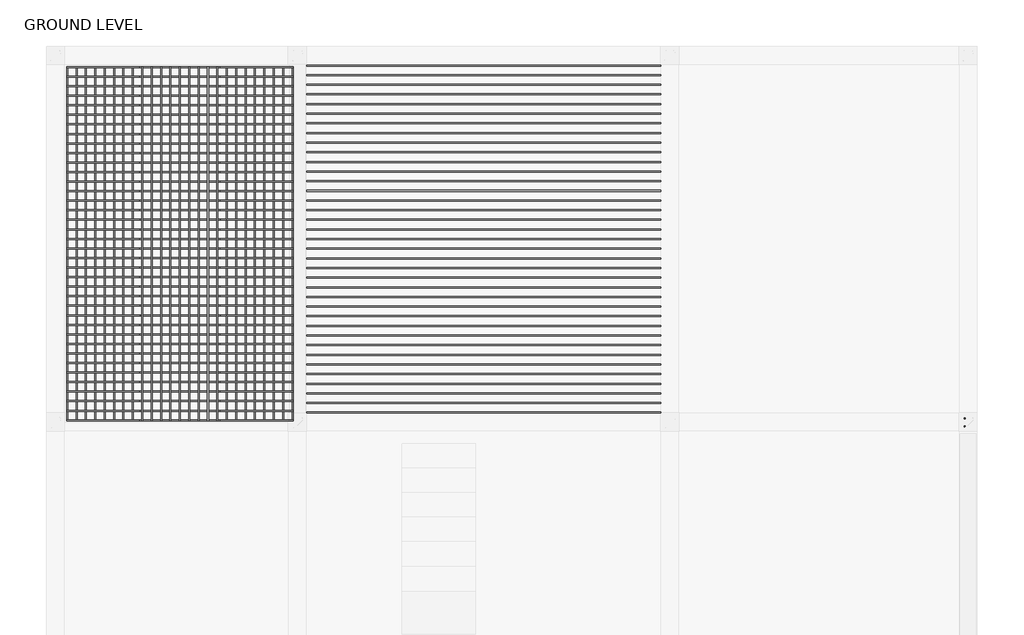
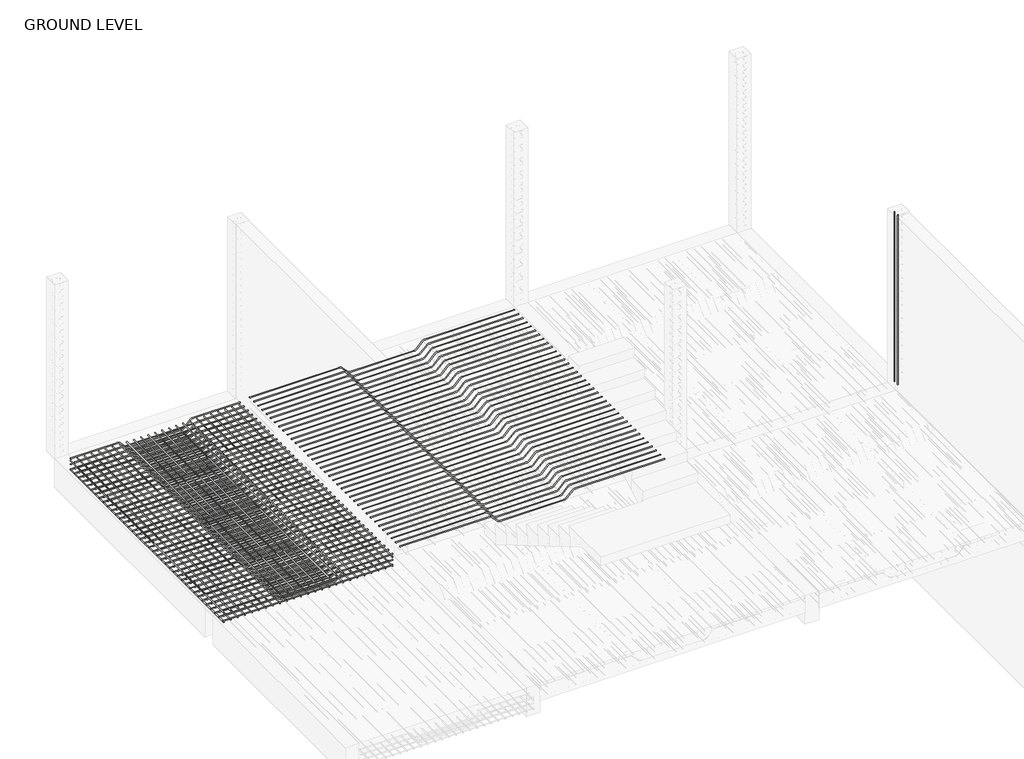
# One storey, part 6 of 8: 7 reinforcing bars.
"""IFC4 building model written with IfcOpenShell, lengths in millimetres."""

from ifc_helpers import new_model, si_unit, point, frame, origin, place, context, project, spatial, polyline, circle_curve, trimmed, segment, composite_curve, source, transform, mapped, element, save
from ifc_brep_helpers import swept_disk

model = new_model("IFC4")

# Units and contexts
model_context = context("Model", 3, world=origin())
ifc_project = project(units=[si_unit("LENGTHUNIT", "METRE", prefix="MILLI")], contexts=[model_context])

# Site, building, storey
site = spatial("IfcSite", under=ifc_project)
building = spatial("IfcBuilding", under=site)
storey = spatial("IfcBuildingStorey", under=building, Name="GROUND LEVEL", Elevation=0.0)

# Reinforcing bars
placement = place(None, origin())
reinforcing_bar_shape = source(origin(), model_context, "Body", "SolidModel", [
    swept_disk(composite_curve([segment(polyline([(-14789.4556799, 4171.9516651, -60.0), (-14008.6544785, 4171.9516651, -60.0)]), True, "CONTINUOUS"), segment(trimmed(circle_curve(frame((-14008.6544785, 4171.9516651, -106.35), z_axis=(0.0, 1.0, 0.0), x_axis=(0.0, 0.0, 46.349999999999994)), 46.35), [point((-14008.6544785, 4171.9516651, -60.0))], [point((-13975.8800792, 4171.9516651, -73.5756007))], True, "CARTESIAN"), True, "CONTINUOUS"), segment(polyline([(-13975.8800792, 4171.9516651, -73.5756007), (-13861.6099243, 4171.9516651, -187.8457555)]), True, "CONTINUOUS"), segment(trimmed(circle_curve(frame((-13828.835525, 4171.9516651, -155.0713562), z_axis=(0.0, -1.0, 0.0), x_axis=(-32.77439930000037, 0.0, -32.7743993)), 46.35), [point((-13861.6099243, 4171.9516651, -187.8457555))], [point((-13828.835525, 4171.9516651, -201.4213562))], True, "CARTESIAN"), True, "CONTINUOUS"), segment(polyline([(-13828.835525, 4171.9516651, -201.4213562), (-12945.2758347, 4171.9516651, -201.4213562)]), True, "CONTINUOUS"), segment(trimmed(circle_curve(frame((-12945.2758347, 4171.9516651, -155.0713562), z_axis=(0.0, -1.0, 0.0), x_axis=(0.0, 0.0, -46.349999999999994)), 46.35), [point((-12945.2758347, 4171.9516651, -201.4213562))], [point((-12912.5014354, 4171.9516651, -187.8457555))], True, "CARTESIAN"), True, "CONTINUOUS"), segment(polyline([(-12912.5014354, 4171.9516651, -187.8457555), (-12798.2312806, 4171.9516651, -73.5756007)]), True, "CONTINUOUS"), segment(trimmed(circle_curve(frame((-12765.4568813, 4171.9516651, -106.35), z_axis=(0.0, 1.0000000000000002, 0.0), x_axis=(-32.77439930000037, 0.0, 32.7743993)), 46.35), [point((-12798.2312806, 4171.9516651, -73.5756007))], [point((-12765.4568813, 4171.9516651, -60.0))], True, "CARTESIAN"), True, "CONTINUOUS"), segment(polyline([(-12765.4568813, 4171.9516651, -60.0), (-11984.6556799, 4171.9516651, -60.0)]), True, "CONTINUOUS")], self_intersect=False), 6.35),
])
element("IfcReinforcingBar", 1, at=placement, inside=storey, context=model_context, shape_type="MappedRepresentation", body=[
    mapped(reinforcing_bar_shape, transform((0.0, 0.0, 0.0), x_axis=(1.0, 0.0, 0.0), y_axis=(0.0, 1.0, 0.0), z_axis=(0.0, 0.0, 1.0))),
    mapped(reinforcing_bar_shape, transform((0.0, -118.3325458, 0.0), x_axis=(1.0, 0.0, 0.0), y_axis=(0.0, 1.0, 0.0), z_axis=(0.0, 0.0, 1.0))),
    mapped(reinforcing_bar_shape, transform((0.0, -236.6650915, 0.0), x_axis=(1.0, 0.0, 0.0), y_axis=(0.0, 1.0, 0.0), z_axis=(0.0, 0.0, 1.0))),
    mapped(reinforcing_bar_shape, transform((0.0, -354.9976373, 0.0), x_axis=(1.0, 0.0, 0.0), y_axis=(0.0, 1.0, 0.0), z_axis=(0.0, 0.0, 1.0))),
    mapped(reinforcing_bar_shape, transform((0.0, -473.330183, 0.0), x_axis=(1.0, 0.0, 0.0), y_axis=(0.0, 1.0, 0.0), z_axis=(0.0, 0.0, 1.0))),
    mapped(reinforcing_bar_shape, transform((0.0, -591.6627288, 0.0), x_axis=(1.0, 0.0, 0.0), y_axis=(0.0, 1.0, 0.0), z_axis=(0.0, 0.0, 1.0))),
    mapped(reinforcing_bar_shape, transform((0.0, -709.9952745, 0.0), x_axis=(1.0, 0.0, 0.0), y_axis=(0.0, 1.0, 0.0), z_axis=(0.0, 0.0, 1.0))),
    mapped(reinforcing_bar_shape, transform((0.0, -828.3278203, 0.0), x_axis=(1.0, 0.0, 0.0), y_axis=(0.0, 1.0, 0.0), z_axis=(0.0, 0.0, 1.0))),
    mapped(reinforcing_bar_shape, transform((0.0, -946.660366, 0.0), x_axis=(1.0, 0.0, 0.0), y_axis=(0.0, 1.0, 0.0), z_axis=(0.0, 0.0, 1.0))),
    mapped(reinforcing_bar_shape, transform((0.0, -1064.9929118, 0.0), x_axis=(1.0, 0.0, 0.0), y_axis=(0.0, 1.0, 0.0), z_axis=(0.0, 0.0, 1.0))),
    mapped(reinforcing_bar_shape, transform((0.0, -1183.3254576, 0.0), x_axis=(1.0, 0.0, 0.0), y_axis=(0.0, 1.0, 0.0), z_axis=(0.0, 0.0, 1.0))),
    mapped(reinforcing_bar_shape, transform((0.0, -1301.6580033, 0.0), x_axis=(1.0, 0.0, 0.0), y_axis=(0.0, 1.0, 0.0), z_axis=(0.0, 0.0, 1.0))),
    mapped(reinforcing_bar_shape, transform((0.0, -1419.9905491, 0.0), x_axis=(1.0, 0.0, 0.0), y_axis=(0.0, 1.0, 0.0), z_axis=(0.0, 0.0, 1.0))),
    mapped(reinforcing_bar_shape, transform((0.0, -1538.3230948, 0.0), x_axis=(1.0, 0.0, 0.0), y_axis=(0.0, 1.0, 0.0), z_axis=(0.0, 0.0, 1.0))),
    mapped(reinforcing_bar_shape, transform((0.0, -1656.6556406, 0.0), x_axis=(1.0, 0.0, 0.0), y_axis=(0.0, 1.0, 0.0), z_axis=(0.0, 0.0, 1.0))),
    mapped(reinforcing_bar_shape, transform((0.0, -1774.9881863, 0.0), x_axis=(1.0, 0.0, 0.0), y_axis=(0.0, 1.0, 0.0), z_axis=(0.0, 0.0, 1.0))),
    mapped(reinforcing_bar_shape, transform((0.0, -1893.3207321, 0.0), x_axis=(1.0, 0.0, 0.0), y_axis=(0.0, 1.0, 0.0), z_axis=(0.0, 0.0, 1.0))),
    mapped(reinforcing_bar_shape, transform((0.0, -2011.6532778, 0.0), x_axis=(1.0, 0.0, 0.0), y_axis=(0.0, 1.0, 0.0), z_axis=(0.0, 0.0, 1.0))),
    mapped(reinforcing_bar_shape, transform((0.0, -2129.9858236, 0.0), x_axis=(1.0, 0.0, 0.0), y_axis=(0.0, 1.0, 0.0), z_axis=(0.0, 0.0, 1.0))),
    mapped(reinforcing_bar_shape, transform((0.0, -2248.3183694, 0.0), x_axis=(1.0, 0.0, 0.0), y_axis=(0.0, 1.0, 0.0), z_axis=(0.0, 0.0, 1.0))),
    mapped(reinforcing_bar_shape, transform((0.0, -2366.6509151, 0.0), x_axis=(1.0, 0.0, 0.0), y_axis=(0.0, 1.0, 0.0), z_axis=(0.0, 0.0, 1.0))),
    mapped(reinforcing_bar_shape, transform((0.0, -2484.9834609, 0.0), x_axis=(1.0, 0.0, 0.0), y_axis=(0.0, 1.0, 0.0), z_axis=(0.0, 0.0, 1.0))),
    mapped(reinforcing_bar_shape, transform((0.0, -2603.3160066, 0.0), x_axis=(1.0, 0.0, 0.0), y_axis=(0.0, 1.0, 0.0), z_axis=(0.0, 0.0, 1.0))),
    mapped(reinforcing_bar_shape, transform((0.0, -2721.6485524, 0.0), x_axis=(1.0, 0.0, 0.0), y_axis=(0.0, 1.0, 0.0), z_axis=(0.0, 0.0, 1.0))),
    mapped(reinforcing_bar_shape, transform((0.0, -2839.9810981, 0.0), x_axis=(1.0, 0.0, 0.0), y_axis=(0.0, 1.0, 0.0), z_axis=(0.0, 0.0, 1.0))),
    mapped(reinforcing_bar_shape, transform((0.0, -2958.3136439, 0.0), x_axis=(1.0, 0.0, 0.0), y_axis=(0.0, 1.0, 0.0), z_axis=(0.0, 0.0, 1.0))),
    mapped(reinforcing_bar_shape, transform((0.0, -3076.6461896, 0.0), x_axis=(1.0, 0.0, 0.0), y_axis=(0.0, 1.0, 0.0), z_axis=(0.0, 0.0, 1.0))),
    mapped(reinforcing_bar_shape, transform((0.0, -3194.9787354, 0.0), x_axis=(1.0, 0.0, 0.0), y_axis=(0.0, 1.0, 0.0), z_axis=(0.0, 0.0, 1.0))),
    mapped(reinforcing_bar_shape, transform((0.0, -3313.3112812, 0.0), x_axis=(1.0, 0.0, 0.0), y_axis=(0.0, 1.0, 0.0), z_axis=(0.0, 0.0, 1.0))),
    mapped(reinforcing_bar_shape, transform((0.0, -3431.6438269, 0.0), x_axis=(1.0, 0.0, 0.0), y_axis=(0.0, 1.0, 0.0), z_axis=(0.0, 0.0, 1.0))),
    mapped(reinforcing_bar_shape, transform((0.0, -3549.9763727, 0.0), x_axis=(1.0, 0.0, 0.0), y_axis=(0.0, 1.0, 0.0), z_axis=(0.0, 0.0, 1.0))),
    mapped(reinforcing_bar_shape, transform((0.0, -3668.3089184, 0.0), x_axis=(1.0, 0.0, 0.0), y_axis=(0.0, 1.0, 0.0), z_axis=(0.0, 0.0, 1.0))),
    mapped(reinforcing_bar_shape, transform((0.0, -3786.6414642, 0.0), x_axis=(1.0, 0.0, 0.0), y_axis=(0.0, 1.0, 0.0), z_axis=(0.0, 0.0, 1.0))),
    mapped(reinforcing_bar_shape, transform((0.0, -3904.9740099, 0.0), x_axis=(1.0, 0.0, 0.0), y_axis=(0.0, 1.0, 0.0), z_axis=(0.0, 0.0, 1.0))),
    mapped(reinforcing_bar_shape, transform((0.0, -4023.3065557, 0.0), x_axis=(1.0, 0.0, 0.0), y_axis=(0.0, 1.0, 0.0), z_axis=(0.0, 0.0, 1.0))),
    mapped(reinforcing_bar_shape, transform((0.0, -4141.6391014, 0.0), x_axis=(1.0, 0.0, 0.0), y_axis=(0.0, 1.0, 0.0), z_axis=(0.0, 0.0, 1.0))),
    mapped(reinforcing_bar_shape, transform((0.0, -4259.9716472, 0.0), x_axis=(1.0, 0.0, 0.0), y_axis=(0.0, 1.0, 0.0), z_axis=(0.0, 0.0, 1.0))),
    mapped(reinforcing_bar_shape, transform((0.0, -4378.304193, 0.0), x_axis=(1.0, 0.0, 0.0), y_axis=(0.0, 1.0, 0.0), z_axis=(0.0, 0.0, 1.0))),
])
reinforcing_bar_2_shape = source(origin(), model_context, "Body", "SolidModel", [
    swept_disk(composite_curve([segment(polyline([(-11984.6556799, 4171.9516651, -249.9712592), (-14789.4556799, 4171.9516651, -249.9712592)]), True, "CONTINUOUS")], self_intersect=False), 6.35),
])
element("IfcReinforcingBar", 2, at=placement, inside=storey, context=model_context, shape_type="MappedRepresentation", body=[
    mapped(reinforcing_bar_2_shape, transform((0.0, 0.0, 0.0), x_axis=(1.0, 0.0, 0.0), y_axis=(0.0, 1.0, 0.0), z_axis=(0.0, 0.0, 1.0))),
    mapped(reinforcing_bar_2_shape, transform((0.0, -118.3325458, 0.0), x_axis=(1.0, 0.0, 0.0), y_axis=(0.0, 1.0, 0.0), z_axis=(0.0, 0.0, 1.0))),
    mapped(reinforcing_bar_2_shape, transform((0.0, -236.6650915, 0.0), x_axis=(1.0, 0.0, 0.0), y_axis=(0.0, 1.0, 0.0), z_axis=(0.0, 0.0, 1.0))),
    mapped(reinforcing_bar_2_shape, transform((0.0, -354.9976373, 0.0), x_axis=(1.0, 0.0, 0.0), y_axis=(0.0, 1.0, 0.0), z_axis=(0.0, 0.0, 1.0))),
    mapped(reinforcing_bar_2_shape, transform((0.0, -473.330183, 0.0), x_axis=(1.0, 0.0, 0.0), y_axis=(0.0, 1.0, 0.0), z_axis=(0.0, 0.0, 1.0))),
    mapped(reinforcing_bar_2_shape, transform((0.0, -591.6627288, 0.0), x_axis=(1.0, 0.0, 0.0), y_axis=(0.0, 1.0, 0.0), z_axis=(0.0, 0.0, 1.0))),
    mapped(reinforcing_bar_2_shape, transform((0.0, -709.9952745, 0.0), x_axis=(1.0, 0.0, 0.0), y_axis=(0.0, 1.0, 0.0), z_axis=(0.0, 0.0, 1.0))),
    mapped(reinforcing_bar_2_shape, transform((0.0, -828.3278203, 0.0), x_axis=(1.0, 0.0, 0.0), y_axis=(0.0, 1.0, 0.0), z_axis=(0.0, 0.0, 1.0))),
    mapped(reinforcing_bar_2_shape, transform((0.0, -946.660366, 0.0), x_axis=(1.0, 0.0, 0.0), y_axis=(0.0, 1.0, 0.0), z_axis=(0.0, 0.0, 1.0))),
    mapped(reinforcing_bar_2_shape, transform((0.0, -1064.9929118, 0.0), x_axis=(1.0, 0.0, 0.0), y_axis=(0.0, 1.0, 0.0), z_axis=(0.0, 0.0, 1.0))),
    mapped(reinforcing_bar_2_shape, transform((0.0, -1183.3254576, 0.0), x_axis=(1.0, 0.0, 0.0), y_axis=(0.0, 1.0, 0.0), z_axis=(0.0, 0.0, 1.0))),
    mapped(reinforcing_bar_2_shape, transform((0.0, -1301.6580033, 0.0), x_axis=(1.0, 0.0, 0.0), y_axis=(0.0, 1.0, 0.0), z_axis=(0.0, 0.0, 1.0))),
    mapped(reinforcing_bar_2_shape, transform((0.0, -1419.9905491, 0.0), x_axis=(1.0, 0.0, 0.0), y_axis=(0.0, 1.0, 0.0), z_axis=(0.0, 0.0, 1.0))),
    mapped(reinforcing_bar_2_shape, transform((0.0, -1538.3230948, 0.0), x_axis=(1.0, 0.0, 0.0), y_axis=(0.0, 1.0, 0.0), z_axis=(0.0, 0.0, 1.0))),
    mapped(reinforcing_bar_2_shape, transform((0.0, -1656.6556406, 0.0), x_axis=(1.0, 0.0, 0.0), y_axis=(0.0, 1.0, 0.0), z_axis=(0.0, 0.0, 1.0))),
    mapped(reinforcing_bar_2_shape, transform((0.0, -1774.9881863, 0.0), x_axis=(1.0, 0.0, 0.0), y_axis=(0.0, 1.0, 0.0), z_axis=(0.0, 0.0, 1.0))),
    mapped(reinforcing_bar_2_shape, transform((0.0, -1893.3207321, 0.0), x_axis=(1.0, 0.0, 0.0), y_axis=(0.0, 1.0, 0.0), z_axis=(0.0, 0.0, 1.0))),
    mapped(reinforcing_bar_2_shape, transform((0.0, -2011.6532778, 0.0), x_axis=(1.0, 0.0, 0.0), y_axis=(0.0, 1.0, 0.0), z_axis=(0.0, 0.0, 1.0))),
    mapped(reinforcing_bar_2_shape, transform((0.0, -2129.9858236, 0.0), x_axis=(1.0, 0.0, 0.0), y_axis=(0.0, 1.0, 0.0), z_axis=(0.0, 0.0, 1.0))),
    mapped(reinforcing_bar_2_shape, transform((0.0, -2248.3183694, 0.0), x_axis=(1.0, 0.0, 0.0), y_axis=(0.0, 1.0, 0.0), z_axis=(0.0, 0.0, 1.0))),
    mapped(reinforcing_bar_2_shape, transform((0.0, -2366.6509151, 0.0), x_axis=(1.0, 0.0, 0.0), y_axis=(0.0, 1.0, 0.0), z_axis=(0.0, 0.0, 1.0))),
    mapped(reinforcing_bar_2_shape, transform((0.0, -2484.9834609, 0.0), x_axis=(1.0, 0.0, 0.0), y_axis=(0.0, 1.0, 0.0), z_axis=(0.0, 0.0, 1.0))),
    mapped(reinforcing_bar_2_shape, transform((0.0, -2603.3160066, 0.0), x_axis=(1.0, 0.0, 0.0), y_axis=(0.0, 1.0, 0.0), z_axis=(0.0, 0.0, 1.0))),
    mapped(reinforcing_bar_2_shape, transform((0.0, -2721.6485524, 0.0), x_axis=(1.0, 0.0, 0.0), y_axis=(0.0, 1.0, 0.0), z_axis=(0.0, 0.0, 1.0))),
    mapped(reinforcing_bar_2_shape, transform((0.0, -2839.9810981, 0.0), x_axis=(1.0, 0.0, 0.0), y_axis=(0.0, 1.0, 0.0), z_axis=(0.0, 0.0, 1.0))),
    mapped(reinforcing_bar_2_shape, transform((0.0, -2958.3136439, 0.0), x_axis=(1.0, 0.0, 0.0), y_axis=(0.0, 1.0, 0.0), z_axis=(0.0, 0.0, 1.0))),
    mapped(reinforcing_bar_2_shape, transform((0.0, -3076.6461896, 0.0), x_axis=(1.0, 0.0, 0.0), y_axis=(0.0, 1.0, 0.0), z_axis=(0.0, 0.0, 1.0))),
    mapped(reinforcing_bar_2_shape, transform((0.0, -3194.9787354, 0.0), x_axis=(1.0, 0.0, 0.0), y_axis=(0.0, 1.0, 0.0), z_axis=(0.0, 0.0, 1.0))),
    mapped(reinforcing_bar_2_shape, transform((0.0, -3313.3112812, 0.0), x_axis=(1.0, 0.0, 0.0), y_axis=(0.0, 1.0, 0.0), z_axis=(0.0, 0.0, 1.0))),
    mapped(reinforcing_bar_2_shape, transform((0.0, -3431.6438269, 0.0), x_axis=(1.0, 0.0, 0.0), y_axis=(0.0, 1.0, 0.0), z_axis=(0.0, 0.0, 1.0))),
    mapped(reinforcing_bar_2_shape, transform((0.0, -3549.9763727, 0.0), x_axis=(1.0, 0.0, 0.0), y_axis=(0.0, 1.0, 0.0), z_axis=(0.0, 0.0, 1.0))),
    mapped(reinforcing_bar_2_shape, transform((0.0, -3668.3089184, 0.0), x_axis=(1.0, 0.0, 0.0), y_axis=(0.0, 1.0, 0.0), z_axis=(0.0, 0.0, 1.0))),
    mapped(reinforcing_bar_2_shape, transform((0.0, -3786.6414642, 0.0), x_axis=(1.0, 0.0, 0.0), y_axis=(0.0, 1.0, 0.0), z_axis=(0.0, 0.0, 1.0))),
    mapped(reinforcing_bar_2_shape, transform((0.0, -3904.9740099, 0.0), x_axis=(1.0, 0.0, 0.0), y_axis=(0.0, 1.0, 0.0), z_axis=(0.0, 0.0, 1.0))),
    mapped(reinforcing_bar_2_shape, transform((0.0, -4023.3065557, 0.0), x_axis=(1.0, 0.0, 0.0), y_axis=(0.0, 1.0, 0.0), z_axis=(0.0, 0.0, 1.0))),
    mapped(reinforcing_bar_2_shape, transform((0.0, -4141.6391014, 0.0), x_axis=(1.0, 0.0, 0.0), y_axis=(0.0, 1.0, 0.0), z_axis=(0.0, 0.0, 1.0))),
    mapped(reinforcing_bar_2_shape, transform((0.0, -4259.9716472, 0.0), x_axis=(1.0, 0.0, 0.0), y_axis=(0.0, 1.0, 0.0), z_axis=(0.0, 0.0, 1.0))),
    mapped(reinforcing_bar_2_shape, transform((0.0, -4378.304193, 0.0), x_axis=(1.0, 0.0, 0.0), y_axis=(0.0, 1.0, 0.0), z_axis=(0.0, 0.0, 1.0))),
])
reinforcing_bar_3_shape = source(origin(), model_context, "Body", "SolidModel", [
    swept_disk(composite_curve([segment(polyline([(-14789.4556799, 4171.9516651, -161.5623157), (-11984.6556799, 4171.9516651, -161.5623157)]), True, "CONTINUOUS")], self_intersect=False), 6.35),
])
element("IfcReinforcingBar", 3, at=placement, inside=storey, context=model_context, shape_type="MappedRepresentation", body=[
    mapped(reinforcing_bar_3_shape, transform((0.0, 0.0, 0.0), x_axis=(1.0, 0.0, 0.0), y_axis=(0.0, 1.0, 0.0), z_axis=(0.0, 0.0, 1.0))),
    mapped(reinforcing_bar_3_shape, transform((0.0, -118.3325458, 0.0), x_axis=(1.0, 0.0, 0.0), y_axis=(0.0, 1.0, 0.0), z_axis=(0.0, 0.0, 1.0))),
    mapped(reinforcing_bar_3_shape, transform((0.0, -236.6650915, 0.0), x_axis=(1.0, 0.0, 0.0), y_axis=(0.0, 1.0, 0.0), z_axis=(0.0, 0.0, 1.0))),
    mapped(reinforcing_bar_3_shape, transform((0.0, -354.9976373, 0.0), x_axis=(1.0, 0.0, 0.0), y_axis=(0.0, 1.0, 0.0), z_axis=(0.0, 0.0, 1.0))),
    mapped(reinforcing_bar_3_shape, transform((0.0, -473.330183, 0.0), x_axis=(1.0, 0.0, 0.0), y_axis=(0.0, 1.0, 0.0), z_axis=(0.0, 0.0, 1.0))),
    mapped(reinforcing_bar_3_shape, transform((0.0, -591.6627288, 0.0), x_axis=(1.0, 0.0, 0.0), y_axis=(0.0, 1.0, 0.0), z_axis=(0.0, 0.0, 1.0))),
    mapped(reinforcing_bar_3_shape, transform((0.0, -709.9952745, 0.0), x_axis=(1.0, 0.0, 0.0), y_axis=(0.0, 1.0, 0.0), z_axis=(0.0, 0.0, 1.0))),
    mapped(reinforcing_bar_3_shape, transform((0.0, -828.3278203, 0.0), x_axis=(1.0, 0.0, 0.0), y_axis=(0.0, 1.0, 0.0), z_axis=(0.0, 0.0, 1.0))),
    mapped(reinforcing_bar_3_shape, transform((0.0, -946.660366, 0.0), x_axis=(1.0, 0.0, 0.0), y_axis=(0.0, 1.0, 0.0), z_axis=(0.0, 0.0, 1.0))),
    mapped(reinforcing_bar_3_shape, transform((0.0, -1064.9929118, 0.0), x_axis=(1.0, 0.0, 0.0), y_axis=(0.0, 1.0, 0.0), z_axis=(0.0, 0.0, 1.0))),
    mapped(reinforcing_bar_3_shape, transform((0.0, -1183.3254576, 0.0), x_axis=(1.0, 0.0, 0.0), y_axis=(0.0, 1.0, 0.0), z_axis=(0.0, 0.0, 1.0))),
    mapped(reinforcing_bar_3_shape, transform((0.0, -1301.6580033, 0.0), x_axis=(1.0, 0.0, 0.0), y_axis=(0.0, 1.0, 0.0), z_axis=(0.0, 0.0, 1.0))),
    mapped(reinforcing_bar_3_shape, transform((0.0, -1419.9905491, 0.0), x_axis=(1.0, 0.0, 0.0), y_axis=(0.0, 1.0, 0.0), z_axis=(0.0, 0.0, 1.0))),
    mapped(reinforcing_bar_3_shape, transform((0.0, -1538.3230948, 0.0), x_axis=(1.0, 0.0, 0.0), y_axis=(0.0, 1.0, 0.0), z_axis=(0.0, 0.0, 1.0))),
    mapped(reinforcing_bar_3_shape, transform((0.0, -1656.6556406, 0.0), x_axis=(1.0, 0.0, 0.0), y_axis=(0.0, 1.0, 0.0), z_axis=(0.0, 0.0, 1.0))),
    mapped(reinforcing_bar_3_shape, transform((0.0, -1774.9881863, 0.0), x_axis=(1.0, 0.0, 0.0), y_axis=(0.0, 1.0, 0.0), z_axis=(0.0, 0.0, 1.0))),
    mapped(reinforcing_bar_3_shape, transform((0.0, -1893.3207321, 0.0), x_axis=(1.0, 0.0, 0.0), y_axis=(0.0, 1.0, 0.0), z_axis=(0.0, 0.0, 1.0))),
    mapped(reinforcing_bar_3_shape, transform((0.0, -2011.6532778, 0.0), x_axis=(1.0, 0.0, 0.0), y_axis=(0.0, 1.0, 0.0), z_axis=(0.0, 0.0, 1.0))),
    mapped(reinforcing_bar_3_shape, transform((0.0, -2129.9858236, 0.0), x_axis=(1.0, 0.0, 0.0), y_axis=(0.0, 1.0, 0.0), z_axis=(0.0, 0.0, 1.0))),
    mapped(reinforcing_bar_3_shape, transform((0.0, -2248.3183694, 0.0), x_axis=(1.0, 0.0, 0.0), y_axis=(0.0, 1.0, 0.0), z_axis=(0.0, 0.0, 1.0))),
    mapped(reinforcing_bar_3_shape, transform((0.0, -2366.6509151, 0.0), x_axis=(1.0, 0.0, 0.0), y_axis=(0.0, 1.0, 0.0), z_axis=(0.0, 0.0, 1.0))),
    mapped(reinforcing_bar_3_shape, transform((0.0, -2484.9834609, 0.0), x_axis=(1.0, 0.0, 0.0), y_axis=(0.0, 1.0, 0.0), z_axis=(0.0, 0.0, 1.0))),
    mapped(reinforcing_bar_3_shape, transform((0.0, -2603.3160066, 0.0), x_axis=(1.0, 0.0, 0.0), y_axis=(0.0, 1.0, 0.0), z_axis=(0.0, 0.0, 1.0))),
    mapped(reinforcing_bar_3_shape, transform((0.0, -2721.6485524, 0.0), x_axis=(1.0, 0.0, 0.0), y_axis=(0.0, 1.0, 0.0), z_axis=(0.0, 0.0, 1.0))),
    mapped(reinforcing_bar_3_shape, transform((0.0, -2839.9810981, 0.0), x_axis=(1.0, 0.0, 0.0), y_axis=(0.0, 1.0, 0.0), z_axis=(0.0, 0.0, 1.0))),
    mapped(reinforcing_bar_3_shape, transform((0.0, -2958.3136439, 0.0), x_axis=(1.0, 0.0, 0.0), y_axis=(0.0, 1.0, 0.0), z_axis=(0.0, 0.0, 1.0))),
    mapped(reinforcing_bar_3_shape, transform((0.0, -3076.6461896, 0.0), x_axis=(1.0, 0.0, 0.0), y_axis=(0.0, 1.0, 0.0), z_axis=(0.0, 0.0, 1.0))),
    mapped(reinforcing_bar_3_shape, transform((0.0, -3194.9787354, 0.0), x_axis=(1.0, 0.0, 0.0), y_axis=(0.0, 1.0, 0.0), z_axis=(0.0, 0.0, 1.0))),
    mapped(reinforcing_bar_3_shape, transform((0.0, -3313.3112812, 0.0), x_axis=(1.0, 0.0, 0.0), y_axis=(0.0, 1.0, 0.0), z_axis=(0.0, 0.0, 1.0))),
    mapped(reinforcing_bar_3_shape, transform((0.0, -3431.6438269, 0.0), x_axis=(1.0, 0.0, 0.0), y_axis=(0.0, 1.0, 0.0), z_axis=(0.0, 0.0, 1.0))),
    mapped(reinforcing_bar_3_shape, transform((0.0, -3549.9763727, 0.0), x_axis=(1.0, 0.0, 0.0), y_axis=(0.0, 1.0, 0.0), z_axis=(0.0, 0.0, 1.0))),
    mapped(reinforcing_bar_3_shape, transform((0.0, -3668.3089184, 0.0), x_axis=(1.0, 0.0, 0.0), y_axis=(0.0, 1.0, 0.0), z_axis=(0.0, 0.0, 1.0))),
    mapped(reinforcing_bar_3_shape, transform((0.0, -3786.6414642, 0.0), x_axis=(1.0, 0.0, 0.0), y_axis=(0.0, 1.0, 0.0), z_axis=(0.0, 0.0, 1.0))),
    mapped(reinforcing_bar_3_shape, transform((0.0, -3904.9740099, 0.0), x_axis=(1.0, 0.0, 0.0), y_axis=(0.0, 1.0, 0.0), z_axis=(0.0, 0.0, 1.0))),
    mapped(reinforcing_bar_3_shape, transform((0.0, -4023.3065557, 0.0), x_axis=(1.0, 0.0, 0.0), y_axis=(0.0, 1.0, 0.0), z_axis=(0.0, 0.0, 1.0))),
    mapped(reinforcing_bar_3_shape, transform((0.0, -4141.6391014, 0.0), x_axis=(1.0, 0.0, 0.0), y_axis=(0.0, 1.0, 0.0), z_axis=(0.0, 0.0, 1.0))),
    mapped(reinforcing_bar_3_shape, transform((0.0, -4259.9716472, 0.0), x_axis=(1.0, 0.0, 0.0), y_axis=(0.0, 1.0, 0.0), z_axis=(0.0, 0.0, 1.0))),
    mapped(reinforcing_bar_3_shape, transform((0.0, -4378.304193, 0.0), x_axis=(1.0, 0.0, 0.0), y_axis=(0.0, 1.0, 0.0), z_axis=(0.0, 0.0, 1.0))),
])
reinforcing_bar_4_shape = source(origin(), model_context, "Body", "SolidModel", [
    swept_disk(composite_curve([segment(polyline([(-14783.1056799, 4178.3016651, -265.2544844), (-14783.1056799, -212.7025279, -265.2544844)]), True, "CONTINUOUS")], self_intersect=False), 6.35),
])
element("IfcReinforcingBar", 4, at=placement, inside=storey, context=model_context, shape_type="MappedRepresentation", body=[
    mapped(reinforcing_bar_4_shape, transform((0.0, 0.0, 0.0), x_axis=(1.0, 0.0, 0.0), y_axis=(0.0, 1.0, 0.0), z_axis=(0.0, 0.0, 1.0))),
    mapped(reinforcing_bar_4_shape, transform((116.3375, 0.0, 0.0), x_axis=(1.0, 0.0, 0.0), y_axis=(0.0, 1.0, 0.0), z_axis=(0.0, 0.0, 1.0))),
    mapped(reinforcing_bar_4_shape, transform((232.675, 0.0, 0.0), x_axis=(1.0, 0.0, 0.0), y_axis=(0.0, 1.0, 0.0), z_axis=(0.0, 0.0, 1.0))),
    mapped(reinforcing_bar_4_shape, transform((349.0125, 0.0, 0.0), x_axis=(1.0, 0.0, 0.0), y_axis=(0.0, 1.0, 0.0), z_axis=(0.0, 0.0, 1.0))),
    mapped(reinforcing_bar_4_shape, transform((465.35, 0.0, 0.0), x_axis=(1.0, 0.0, 0.0), y_axis=(0.0, 1.0, 0.0), z_axis=(0.0, 0.0, 1.0))),
    mapped(reinforcing_bar_4_shape, transform((581.6875, 0.0, 0.0), x_axis=(1.0, 0.0, 0.0), y_axis=(0.0, 1.0, 0.0), z_axis=(0.0, 0.0, 1.0))),
    mapped(reinforcing_bar_4_shape, transform((698.025, 0.0, 0.0), x_axis=(1.0, 0.0, 0.0), y_axis=(0.0, 1.0, 0.0), z_axis=(0.0, 0.0, 1.0))),
    mapped(reinforcing_bar_4_shape, transform((814.3625, 0.0, 0.0), x_axis=(1.0, 0.0, 0.0), y_axis=(0.0, 1.0, 0.0), z_axis=(0.0, 0.0, 1.0))),
    mapped(reinforcing_bar_4_shape, transform((930.7, 0.0, 0.0), x_axis=(1.0, 0.0, 0.0), y_axis=(0.0, 1.0, 0.0), z_axis=(0.0, 0.0, 1.0))),
    mapped(reinforcing_bar_4_shape, transform((1047.0375, 0.0, 0.0), x_axis=(1.0, 0.0, 0.0), y_axis=(0.0, 1.0, 0.0), z_axis=(0.0, 0.0, 1.0))),
    mapped(reinforcing_bar_4_shape, transform((1163.375, 0.0, 0.0), x_axis=(1.0, 0.0, 0.0), y_axis=(0.0, 1.0, 0.0), z_axis=(0.0, 0.0, 1.0))),
    mapped(reinforcing_bar_4_shape, transform((1279.7125, 0.0, 0.0), x_axis=(1.0, 0.0, 0.0), y_axis=(0.0, 1.0, 0.0), z_axis=(0.0, 0.0, 1.0))),
    mapped(reinforcing_bar_4_shape, transform((1396.05, 0.0, 0.0), x_axis=(1.0, 0.0, 0.0), y_axis=(0.0, 1.0, 0.0), z_axis=(0.0, 0.0, 1.0))),
    mapped(reinforcing_bar_4_shape, transform((1512.3875, 0.0, 0.0), x_axis=(1.0, 0.0, 0.0), y_axis=(0.0, 1.0, 0.0), z_axis=(0.0, 0.0, 1.0))),
    mapped(reinforcing_bar_4_shape, transform((1628.725, 0.0, 0.0), x_axis=(1.0, 0.0, 0.0), y_axis=(0.0, 1.0, 0.0), z_axis=(0.0, 0.0, 1.0))),
    mapped(reinforcing_bar_4_shape, transform((1745.0625, 0.0, 0.0), x_axis=(1.0, 0.0, 0.0), y_axis=(0.0, 1.0, 0.0), z_axis=(0.0, 0.0, 1.0))),
    mapped(reinforcing_bar_4_shape, transform((1861.4, 0.0, 0.0), x_axis=(1.0, 0.0, 0.0), y_axis=(0.0, 1.0, 0.0), z_axis=(0.0, 0.0, 1.0))),
    mapped(reinforcing_bar_4_shape, transform((1977.7375, 0.0, 0.0), x_axis=(1.0, 0.0, 0.0), y_axis=(0.0, 1.0, 0.0), z_axis=(0.0, 0.0, 1.0))),
    mapped(reinforcing_bar_4_shape, transform((2094.075, 0.0, 0.0), x_axis=(1.0, 0.0, 0.0), y_axis=(0.0, 1.0, 0.0), z_axis=(0.0, 0.0, 1.0))),
    mapped(reinforcing_bar_4_shape, transform((2210.4125, 0.0, 0.0), x_axis=(1.0, 0.0, 0.0), y_axis=(0.0, 1.0, 0.0), z_axis=(0.0, 0.0, 1.0))),
    mapped(reinforcing_bar_4_shape, transform((2326.75, 0.0, 0.0), x_axis=(1.0, 0.0, 0.0), y_axis=(0.0, 1.0, 0.0), z_axis=(0.0, 0.0, 1.0))),
    mapped(reinforcing_bar_4_shape, transform((2443.0875, 0.0, 0.0), x_axis=(1.0, 0.0, 0.0), y_axis=(0.0, 1.0, 0.0), z_axis=(0.0, 0.0, 1.0))),
    mapped(reinforcing_bar_4_shape, transform((2559.425, 0.0, 0.0), x_axis=(1.0, 0.0, 0.0), y_axis=(0.0, 1.0, 0.0), z_axis=(0.0, 0.0, 1.0))),
    mapped(reinforcing_bar_4_shape, transform((2675.7625, 0.0, 0.0), x_axis=(1.0, 0.0, 0.0), y_axis=(0.0, 1.0, 0.0), z_axis=(0.0, 0.0, 1.0))),
    mapped(reinforcing_bar_4_shape, transform((2792.1, 0.0, 0.0), x_axis=(1.0, 0.0, 0.0), y_axis=(0.0, 1.0, 0.0), z_axis=(0.0, 0.0, 1.0))),
])
reinforcing_bar_5_shape = source(origin(), model_context, "Body", "SolidModel", [
    swept_disk(composite_curve([segment(polyline([(-14783.1056799, 4178.3016651, -105.2544844), (-14783.1056799, -212.7025279, -105.2544844)]), True, "CONTINUOUS")], self_intersect=False), 6.35),
])
element("IfcReinforcingBar", 5, at=placement, inside=storey, context=model_context, shape_type="MappedRepresentation", body=[
    mapped(reinforcing_bar_5_shape, transform((0.0, 0.0, 0.0), x_axis=(1.0, 0.0, 0.0), y_axis=(0.0, 1.0, 0.0), z_axis=(0.0, 0.0, 1.0))),
    mapped(reinforcing_bar_5_shape, transform((116.3375, 0.0, 0.0), x_axis=(1.0, 0.0, 0.0), y_axis=(0.0, 1.0, 0.0), z_axis=(0.0, 0.0, 1.0))),
    mapped(reinforcing_bar_5_shape, transform((232.675, 0.0, 0.0), x_axis=(1.0, 0.0, 0.0), y_axis=(0.0, 1.0, 0.0), z_axis=(0.0, 0.0, 1.0))),
    mapped(reinforcing_bar_5_shape, transform((349.0125, 0.0, 0.0), x_axis=(1.0, 0.0, 0.0), y_axis=(0.0, 1.0, 0.0), z_axis=(0.0, 0.0, 1.0))),
    mapped(reinforcing_bar_5_shape, transform((465.35, 0.0, 0.0), x_axis=(1.0, 0.0, 0.0), y_axis=(0.0, 1.0, 0.0), z_axis=(0.0, 0.0, 1.0))),
    mapped(reinforcing_bar_5_shape, transform((581.6875, 0.0, 0.0), x_axis=(1.0, 0.0, 0.0), y_axis=(0.0, 1.0, 0.0), z_axis=(0.0, 0.0, 1.0))),
    mapped(reinforcing_bar_5_shape, transform((698.025, 0.0, 0.0), x_axis=(1.0, 0.0, 0.0), y_axis=(0.0, 1.0, 0.0), z_axis=(0.0, 0.0, 1.0))),
    mapped(reinforcing_bar_5_shape, transform((814.3625, 0.0, 0.0), x_axis=(1.0, 0.0, 0.0), y_axis=(0.0, 1.0, 0.0), z_axis=(0.0, 0.0, 1.0))),
    mapped(reinforcing_bar_5_shape, transform((930.7, 0.0, 0.0), x_axis=(1.0, 0.0, 0.0), y_axis=(0.0, 1.0, 0.0), z_axis=(0.0, 0.0, 1.0))),
    mapped(reinforcing_bar_5_shape, transform((1047.0375, 0.0, 0.0), x_axis=(1.0, 0.0, 0.0), y_axis=(0.0, 1.0, 0.0), z_axis=(0.0, 0.0, 1.0))),
    mapped(reinforcing_bar_5_shape, transform((1163.375, 0.0, 0.0), x_axis=(1.0, 0.0, 0.0), y_axis=(0.0, 1.0, 0.0), z_axis=(0.0, 0.0, 1.0))),
    mapped(reinforcing_bar_5_shape, transform((1279.7125, 0.0, 0.0), x_axis=(1.0, 0.0, 0.0), y_axis=(0.0, 1.0, 0.0), z_axis=(0.0, 0.0, 1.0))),
    mapped(reinforcing_bar_5_shape, transform((1396.05, 0.0, 0.0), x_axis=(1.0, 0.0, 0.0), y_axis=(0.0, 1.0, 0.0), z_axis=(0.0, 0.0, 1.0))),
    mapped(reinforcing_bar_5_shape, transform((1512.3875, 0.0, 0.0), x_axis=(1.0, 0.0, 0.0), y_axis=(0.0, 1.0, 0.0), z_axis=(0.0, 0.0, 1.0))),
    mapped(reinforcing_bar_5_shape, transform((1628.725, 0.0, 0.0), x_axis=(1.0, 0.0, 0.0), y_axis=(0.0, 1.0, 0.0), z_axis=(0.0, 0.0, 1.0))),
    mapped(reinforcing_bar_5_shape, transform((1745.0625, 0.0, 0.0), x_axis=(1.0, 0.0, 0.0), y_axis=(0.0, 1.0, 0.0), z_axis=(0.0, 0.0, 1.0))),
    mapped(reinforcing_bar_5_shape, transform((1861.4, 0.0, 0.0), x_axis=(1.0, 0.0, 0.0), y_axis=(0.0, 1.0, 0.0), z_axis=(0.0, 0.0, 1.0))),
    mapped(reinforcing_bar_5_shape, transform((1977.7375, 0.0, 0.0), x_axis=(1.0, 0.0, 0.0), y_axis=(0.0, 1.0, 0.0), z_axis=(0.0, 0.0, 1.0))),
    mapped(reinforcing_bar_5_shape, transform((2094.075, 0.0, 0.0), x_axis=(1.0, 0.0, 0.0), y_axis=(0.0, 1.0, 0.0), z_axis=(0.0, 0.0, 1.0))),
    mapped(reinforcing_bar_5_shape, transform((2210.4125, 0.0, 0.0), x_axis=(1.0, 0.0, 0.0), y_axis=(0.0, 1.0, 0.0), z_axis=(0.0, 0.0, 1.0))),
    mapped(reinforcing_bar_5_shape, transform((2326.75, 0.0, 0.0), x_axis=(1.0, 0.0, 0.0), y_axis=(0.0, 1.0, 0.0), z_axis=(0.0, 0.0, 1.0))),
    mapped(reinforcing_bar_5_shape, transform((2443.0875, 0.0, 0.0), x_axis=(1.0, 0.0, 0.0), y_axis=(0.0, 1.0, 0.0), z_axis=(0.0, 0.0, 1.0))),
    mapped(reinforcing_bar_5_shape, transform((2559.425, 0.0, 0.0), x_axis=(1.0, 0.0, 0.0), y_axis=(0.0, 1.0, 0.0), z_axis=(0.0, 0.0, 1.0))),
    mapped(reinforcing_bar_5_shape, transform((2675.7625, 0.0, 0.0), x_axis=(1.0, 0.0, 0.0), y_axis=(0.0, 1.0, 0.0), z_axis=(0.0, 0.0, 1.0))),
    mapped(reinforcing_bar_5_shape, transform((2792.1, 0.0, 0.0), x_axis=(1.0, 0.0, 0.0), y_axis=(0.0, 1.0, 0.0), z_axis=(0.0, 0.0, 1.0))),
])
reinforcing_bar_6_shape = source(origin(), model_context, "Body", "SolidModel", [
    swept_disk(composite_curve([segment(polyline([(-11812.2556799, 4191.9516645, -46.35), (-10325.9161368, 4191.9516645, -46.35)]), True, "CONTINUOUS"), segment(trimmed(circle_curve(frame((-10325.9161368, 4191.9516645, -92.7), z_axis=(0.0, 1.0, 0.0), x_axis=(0.0, 0.0, 46.35)), 46.35), [point((-10325.9161368, 4191.9516645, -46.35))], [point((-10293.1417375, 4191.9516645, -59.9256007))], True, "CARTESIAN"), True, "CONTINUOUS"), segment(polyline([(-10293.1417375, 4191.9516645, -59.9256007), (-10185.2215826, 4191.9516645, -167.8457555)]), True, "CONTINUOUS"), segment(trimmed(circle_curve(frame((-10152.4471833, 4191.9516645, -135.0713562), z_axis=(0.0, -1.0, 0.0), x_axis=(-32.77439929999855, 0.0, -32.7743993)), 46.35), [point((-10185.2215826, 4191.9516645, -167.8457555))], [point((-10152.4471833, 4191.9516645, -181.4213562))], True, "CARTESIAN"), True, "CONTINUOUS"), segment(polyline([(-10152.4471833, 4191.9516645, -181.4213562), (-9088.5758347, 4191.9516645, -181.4213562)]), True, "CONTINUOUS"), segment(trimmed(circle_curve(frame((-9088.5758347, 4191.9516645, -135.0713562), z_axis=(0.0, -1.0, 0.0), x_axis=(0.0, 0.0, -46.349999999999994)), 46.35), [point((-9088.5758347, 4191.9516645, -181.4213562))], [point((-9055.8014354, 4191.9516645, -167.8457555))], True, "CARTESIAN"), True, "CONTINUOUS"), segment(polyline([(-9055.8014354, 4191.9516645, -167.8457555), (-8947.8812806, 4191.9516645, -59.9256007)]), True, "CONTINUOUS"), segment(trimmed(circle_curve(frame((-8915.1068813, 4191.9516645, -92.7), z_axis=(0.0, 1.0, 0.0), x_axis=(-32.77439930000037, 0.0, 32.774399300000006)), 46.35), [point((-8947.8812806, 4191.9516645, -59.9256007))], [point((-8915.1068813, 4191.9516645, -46.35))], True, "CARTESIAN"), True, "CONTINUOUS"), segment(polyline([(-8915.1068813, 4191.9516645, -46.35), (-7428.7673382, 4191.9516645, -46.35)]), True, "CONTINUOUS")], self_intersect=False), 6.35),
])
element("IfcReinforcingBar", 6, at=placement, inside=storey, context=model_context, shape_type="MappedRepresentation", body=[
    mapped(reinforcing_bar_6_shape, transform((0.0, 0.0, 0.0), x_axis=(1.0, 0.0, 0.0), y_axis=(0.0, 1.0, 0.0), z_axis=(0.0, 0.0, 1.0))),
    mapped(reinforcing_bar_6_shape, transform((0.0, -119.555672, 0.0), x_axis=(1.0, 0.0, 0.0), y_axis=(0.0, 1.0, 0.0), z_axis=(0.0, 0.0, 1.0))),
    mapped(reinforcing_bar_6_shape, transform((0.0, -239.111344, 0.0), x_axis=(1.0, 0.0, 0.0), y_axis=(0.0, 1.0, 0.0), z_axis=(0.0, 0.0, 1.0))),
    mapped(reinforcing_bar_6_shape, transform((0.0, -358.667016, 0.0), x_axis=(1.0, 0.0, 0.0), y_axis=(0.0, 1.0, 0.0), z_axis=(0.0, 0.0, 1.0))),
    mapped(reinforcing_bar_6_shape, transform((0.0, -478.222688, 0.0), x_axis=(1.0, 0.0, 0.0), y_axis=(0.0, 1.0, 0.0), z_axis=(0.0, 0.0, 1.0))),
    mapped(reinforcing_bar_6_shape, transform((0.0, -597.77836, 0.0), x_axis=(1.0, 0.0, 0.0), y_axis=(0.0, 1.0, 0.0), z_axis=(0.0, 0.0, 1.0))),
    mapped(reinforcing_bar_6_shape, transform((0.0, -717.3340321, 0.0), x_axis=(1.0, 0.0, 0.0), y_axis=(0.0, 1.0, 0.0), z_axis=(0.0, 0.0, 1.0))),
    mapped(reinforcing_bar_6_shape, transform((0.0, -836.8897041, 0.0), x_axis=(1.0, 0.0, 0.0), y_axis=(0.0, 1.0, 0.0), z_axis=(0.0, 0.0, 1.0))),
    mapped(reinforcing_bar_6_shape, transform((0.0, -956.4453761, 0.0), x_axis=(1.0, 0.0, 0.0), y_axis=(0.0, 1.0, 0.0), z_axis=(0.0, 0.0, 1.0))),
    mapped(reinforcing_bar_6_shape, transform((0.0, -1076.0010481, 0.0), x_axis=(1.0, 0.0, 0.0), y_axis=(0.0, 1.0, 0.0), z_axis=(0.0, 0.0, 1.0))),
    mapped(reinforcing_bar_6_shape, transform((0.0, -1195.5567201, 0.0), x_axis=(1.0, 0.0, 0.0), y_axis=(0.0, 1.0, 0.0), z_axis=(0.0, 0.0, 1.0))),
    mapped(reinforcing_bar_6_shape, transform((0.0, -1315.1123921, 0.0), x_axis=(1.0, 0.0, 0.0), y_axis=(0.0, 1.0, 0.0), z_axis=(0.0, 0.0, 1.0))),
    mapped(reinforcing_bar_6_shape, transform((0.0, -1434.6680641, 0.0), x_axis=(1.0, 0.0, 0.0), y_axis=(0.0, 1.0, 0.0), z_axis=(0.0, 0.0, 1.0))),
    mapped(reinforcing_bar_6_shape, transform((0.0, -1554.2237361, 0.0), x_axis=(1.0, 0.0, 0.0), y_axis=(0.0, 1.0, 0.0), z_axis=(0.0, 0.0, 1.0))),
    mapped(reinforcing_bar_6_shape, transform((0.0, -1673.7794081, 0.0), x_axis=(1.0, 0.0, 0.0), y_axis=(0.0, 1.0, 0.0), z_axis=(0.0, 0.0, 1.0))),
    mapped(reinforcing_bar_6_shape, transform((0.0, -1793.3350801, 0.0), x_axis=(1.0, 0.0, 0.0), y_axis=(0.0, 1.0, 0.0), z_axis=(0.0, 0.0, 1.0))),
    mapped(reinforcing_bar_6_shape, transform((0.0, -1912.8907522, 0.0), x_axis=(1.0, 0.0, 0.0), y_axis=(0.0, 1.0, 0.0), z_axis=(0.0, 0.0, 1.0))),
    mapped(reinforcing_bar_6_shape, transform((0.0, -2032.4464242, 0.0), x_axis=(1.0, 0.0, 0.0), y_axis=(0.0, 1.0, 0.0), z_axis=(0.0, 0.0, 1.0))),
    mapped(reinforcing_bar_6_shape, transform((0.0, -2152.0020962, 0.0), x_axis=(1.0, 0.0, 0.0), y_axis=(0.0, 1.0, 0.0), z_axis=(0.0, 0.0, 1.0))),
    mapped(reinforcing_bar_6_shape, transform((0.0, -2271.5577682, 0.0), x_axis=(1.0, 0.0, 0.0), y_axis=(0.0, 1.0, 0.0), z_axis=(0.0, 0.0, 1.0))),
    mapped(reinforcing_bar_6_shape, transform((0.0, -2391.1134402, 0.0), x_axis=(1.0, 0.0, 0.0), y_axis=(0.0, 1.0, 0.0), z_axis=(0.0, 0.0, 1.0))),
    mapped(reinforcing_bar_6_shape, transform((0.0, -2510.6691122, 0.0), x_axis=(1.0, 0.0, 0.0), y_axis=(0.0, 1.0, 0.0), z_axis=(0.0, 0.0, 1.0))),
    mapped(reinforcing_bar_6_shape, transform((0.0, -2630.2247842, 0.0), x_axis=(1.0, 0.0, 0.0), y_axis=(0.0, 1.0, 0.0), z_axis=(0.0, 0.0, 1.0))),
    mapped(reinforcing_bar_6_shape, transform((0.0, -2749.7804562, 0.0), x_axis=(1.0, 0.0, 0.0), y_axis=(0.0, 1.0, 0.0), z_axis=(0.0, 0.0, 1.0))),
    mapped(reinforcing_bar_6_shape, transform((0.0, -2869.3361282, 0.0), x_axis=(1.0, 0.0, 0.0), y_axis=(0.0, 1.0, 0.0), z_axis=(0.0, 0.0, 1.0))),
    mapped(reinforcing_bar_6_shape, transform((0.0, -2988.8918002, 0.0), x_axis=(1.0, 0.0, 0.0), y_axis=(0.0, 1.0, 0.0), z_axis=(0.0, 0.0, 1.0))),
    mapped(reinforcing_bar_6_shape, transform((0.0, -3108.4474723, 0.0), x_axis=(1.0, 0.0, 0.0), y_axis=(0.0, 1.0, 0.0), z_axis=(0.0, 0.0, 1.0))),
    mapped(reinforcing_bar_6_shape, transform((0.0, -3228.0031443, 0.0), x_axis=(1.0, 0.0, 0.0), y_axis=(0.0, 1.0, 0.0), z_axis=(0.0, 0.0, 1.0))),
    mapped(reinforcing_bar_6_shape, transform((0.0, -3347.5588163, 0.0), x_axis=(1.0, 0.0, 0.0), y_axis=(0.0, 1.0, 0.0), z_axis=(0.0, 0.0, 1.0))),
    mapped(reinforcing_bar_6_shape, transform((0.0, -3467.1144883, 0.0), x_axis=(1.0, 0.0, 0.0), y_axis=(0.0, 1.0, 0.0), z_axis=(0.0, 0.0, 1.0))),
    mapped(reinforcing_bar_6_shape, transform((0.0, -3586.6701603, 0.0), x_axis=(1.0, 0.0, 0.0), y_axis=(0.0, 1.0, 0.0), z_axis=(0.0, 0.0, 1.0))),
    mapped(reinforcing_bar_6_shape, transform((0.0, -3706.2258323, 0.0), x_axis=(1.0, 0.0, 0.0), y_axis=(0.0, 1.0, 0.0), z_axis=(0.0, 0.0, 1.0))),
    mapped(reinforcing_bar_6_shape, transform((0.0, -3825.7815043, 0.0), x_axis=(1.0, 0.0, 0.0), y_axis=(0.0, 1.0, 0.0), z_axis=(0.0, 0.0, 1.0))),
    mapped(reinforcing_bar_6_shape, transform((0.0, -3945.3371763, 0.0), x_axis=(1.0, 0.0, 0.0), y_axis=(0.0, 1.0, 0.0), z_axis=(0.0, 0.0, 1.0))),
    mapped(reinforcing_bar_6_shape, transform((0.0, -4064.8928483, 0.0), x_axis=(1.0, 0.0, 0.0), y_axis=(0.0, 1.0, 0.0), z_axis=(0.0, 0.0, 1.0))),
    mapped(reinforcing_bar_6_shape, transform((0.0, -4184.4485203, 0.0), x_axis=(1.0, 0.0, 0.0), y_axis=(0.0, 1.0, 0.0), z_axis=(0.0, 0.0, 1.0))),
    mapped(reinforcing_bar_6_shape, transform((0.0, -4304.0041923, 0.0), x_axis=(1.0, 0.0, 0.0), y_axis=(0.0, 1.0, 0.0), z_axis=(0.0, 0.0, 1.0))),
])
reinforcing_bar_7_shape = source(origin(), model_context, "Body", "SolidModel", [
    swept_disk(composite_curve([segment(polyline([(-3665.5106662, -183.9048321, 3008.0), (-3665.5106662, -183.9048321, 40.0)]), True, "CONTINUOUS")], self_intersect=False), 6.35),
])
element("IfcReinforcingBar", 7, at=placement, inside=storey, context=model_context, shape_type="MappedRepresentation", body=[
    mapped(reinforcing_bar_7_shape, transform((0.0, 0.0, 0.0), x_axis=(1.0, 0.0, 0.0), y_axis=(0.0, 1.0, 0.0), z_axis=(0.0, 0.0, 1.0))),
    mapped(reinforcing_bar_7_shape, transform((0.0, -96.9916148, 0.0), x_axis=(1.0, 0.0, 0.0), y_axis=(0.0, 1.0, 0.0), z_axis=(0.0, 0.0, 1.0))),
])

save(model, "model.ifc")

# Revit data of these elements
# Elements 1, 2, 3, 4, 5, 6, 7 (IfcReinforcingBar)
#   Phase Created = New Construction
